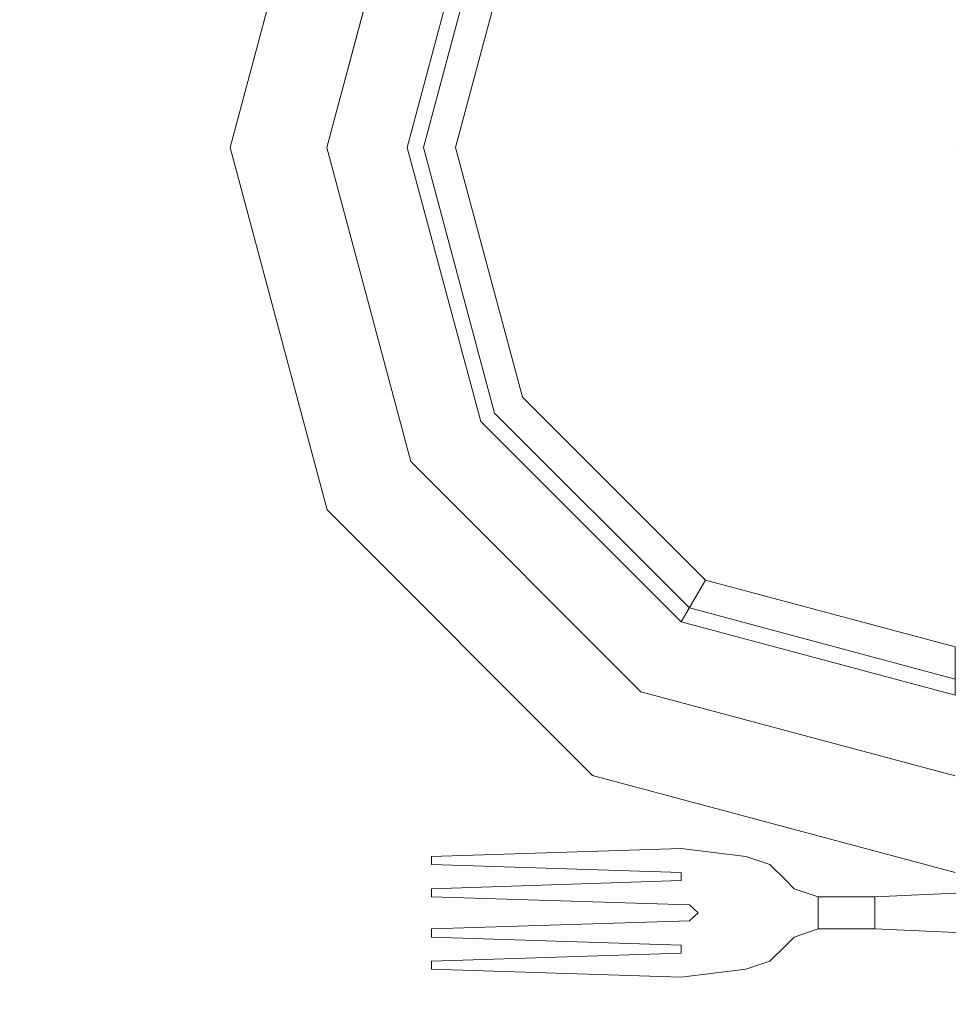
# Model space of a CAD drawing. Units: inches. Extents: x 375 to 1122, y 27 to 1069.
# Tile 55 of 155: x 732.625 to 739.718, y 296.542 to 304.063. Entities that reach past the tile are written whole.
import ezdxf

# ---------------------------------------------------------------- set-up
doc = ezdxf.new("R2010")
doc.units = ezdxf.units.IN
doc.layers.add('A-ANNO-DIMS', color=2, linetype='Continuous', lineweight=18)
doc.layers.add('Furniture', color=30, linetype='Continuous', lineweight=18)
doc.styles.get("Standard").update_dxf_attribs({"font": 'arial.ttf'})
doc.dimstyles.new('ISO-25', dxfattribs={"dimtxt": 12, "dimasz": 2.5, "dimexe": 1.5, "dimexo": 1.5, "dimtad": 1, "dimdec": 1, "dimlunit": 3, "dimtxsty": 'Standard', "dimblk": 'ARCHTICK', "dimcen": 2.5, "dimadec": 0, "dimazin": 0, "dimtfac": 1, "dimtdec": 1, "dimtmove": 0, "dimatfit": 3, "dimfxl": 1.5, "dimfxlon": 1, "dimarcsym": 0})

# ---------------------------------------------------------------- blocks, each defined once
blk = doc.blocks.new('A$C403C54AD')
for p, q in [((1.2372, 1.33067, -0.03581), (1.23566, 1.33529, -0.03534)), ((1.2372, 1.33067, -0.03888), (1.23566, 1.33529, -0.03842))]:
    blk.add_line(p, q)
for points, invisible_edges in [([(1.22181, 1.3907, -0.03153), (1.23105, 1.3907, -0.03153), (1.22951, 1.3553, -0.02863), (1.22335, 1.3553, -0.02863)], 1), ([(1.22181, 1.3907, -0.03153), (1.22181, 1.3907, -0.03461), (1.22335, 1.3553, -0.03122), (1.22335, 1.3553, -0.02863)], 5), ([(1.22181, 1.3907, -0.03461), (1.23105, 1.3907, -0.03461), (1.22951, 1.3553, -0.03122), (1.22335, 1.3553, -0.03122)], 1), ([(1.22951, 1.3553, -0.02863), (1.22951, 1.3553, -0.03122), (1.23105, 1.3907, -0.03461), (1.23105, 1.3907, -0.03153)], 5), ([(1.22335, 1.3553, -0.03122), (1.22335, 1.3553, -0.02863), (1.22335, 1.34452, -0.03071), (1.22335, 1.34452, -0.0333)], 5), ([(1.22951, 1.34452, -0.0333), (1.22951, 1.34452, -0.03071), (1.22951, 1.3553, -0.02863), (1.22951, 1.3553, -0.03122)], 5), ([(1.22335, 1.34452, -0.03071), (1.22951, 1.34452, -0.03071), (1.23105, 1.33991, -0.03306), (1.22181, 1.33991, -0.03306)], 4), ([(1.22335, 1.34452, -0.03071), (1.22335, 1.34452, -0.0333), (1.22181, 1.33991, -0.03584), (1.22181, 1.33991, -0.03306)], 5), ([(1.22335, 1.34452, -0.0333), (1.22951, 1.34452, -0.0333), (1.23105, 1.33991, -0.03584), (1.22181, 1.33991, -0.03584)], 4), ([(1.22951, 1.34452, -0.0333), (1.22951, 1.34452, -0.03071), (1.23105, 1.33991, -0.03306), (1.23105, 1.33991, -0.03584)], 5), ([(1.23105, 1.33991, -0.03306), (1.22181, 1.33991, -0.03306), (1.22027, 1.33837, -0.0341), (1.23258, 1.33837, -0.0341)], 5), ([(1.23105, 1.33991, -0.03584), (1.22181, 1.33991, -0.03584), (1.22027, 1.33837, -0.03718), (1.23258, 1.33837, -0.03718)], 5), ([(1.22181, 1.33991, -0.03584), (1.22181, 1.33991, -0.03306), (1.22027, 1.33837, -0.0341), (1.22027, 1.33837, -0.03718)], 1), ([(1.23105, 1.33991, -0.03306), (1.23105, 1.33991, -0.03584), (1.23258, 1.33837, -0.03718), (1.23258, 1.33837, -0.0341)], 1), ([(1.23258, 1.33837, -0.03718), (1.22027, 1.33837, -0.03718), (1.21719, 1.33529, -0.03842), (1.23566, 1.33529, -0.03842)], 5), ([(1.23258, 1.33837, -0.0341), (1.22027, 1.33837, -0.0341), (1.21719, 1.33529, -0.03534), (1.23566, 1.33529, -0.03534)], 5), ([(1.21719, 1.33529, -0.03534), (1.23566, 1.33529, -0.03534), (1.2372, 1.33067, -0.03581), (1.21565, 1.33067, -0.03581)], 5), ([(1.21719, 1.33529, -0.03842), (1.23566, 1.33529, -0.03842), (1.2372, 1.33067, -0.03888), (1.21565, 1.33067, -0.03888)], 5), ([(1.21719, 1.33529, -0.03842), (1.21719, 1.33529, -0.03534), (1.21565, 1.33067, -0.03581), (1.21565, 1.33067, -0.03888)], 4), ([(1.23566, 1.33529, -0.03534), (1.23566, 1.33529, -0.03842), (1.2372, 1.33067, -0.03888), (1.2372, 1.33067, -0.03581)], 4), ([(1.21565, 1.33067, -0.03581), (1.22027, 1.31836, -0.03521), (1.21873, 1.31836, -0.03521), (1.21411, 1.31836, -0.03521)], 5), ([(1.21565, 1.33067, -0.03888), (1.22027, 1.31836, -0.03829), (1.21873, 1.31836, -0.03829), (1.21411, 1.31836, -0.03829)], 5), ([(1.21565, 1.33067, -0.03581), (1.21565, 1.33067, -0.03888), (1.21411, 1.31836, -0.03829), (1.21411, 1.31836, -0.03521)], 1), ([(1.21565, 1.33067, -0.03581), (1.22643, 1.32156, -0.0356), (1.22489, 1.3199, -0.03545), (1.22027, 1.31836, -0.03521)], 13), ([(1.21565, 1.33067, -0.03581), (1.22643, 1.32156, -0.0356), (1.2372, 1.33067, -0.03581), (1.21565, 1.33067, -0.03581)], 7), ([(1.21565, 1.33067, -0.03888), (1.22643, 1.32156, -0.03868), (1.2372, 1.33067, -0.03888), (1.21565, 1.33067, -0.03888)], 7), ([(1.21565, 1.33067, -0.03888), (1.22643, 1.32156, -0.03868), (1.22489, 1.3199, -0.03853), (1.22027, 1.31836, -0.03829)], 13), ([(1.2372, 1.33067, -0.03581), (1.22643, 1.32156, -0.0356), (1.22797, 1.3199, -0.03545), (1.23258, 1.31836, -0.03521)], 13), ([(1.2372, 1.33067, -0.03888), (1.22643, 1.32156, -0.03868), (1.22797, 1.3199, -0.03853), (1.23258, 1.31836, -0.03829)], 13), ([(1.2372, 1.33067, -0.03581), (1.23258, 1.31836, -0.03521), (1.23412, 1.31836, -0.03521), (1.23874, 1.31836, -0.03521)], 5), ([(1.2372, 1.33067, -0.03888), (1.23258, 1.31836, -0.03829), (1.23412, 1.31836, -0.03829), (1.23874, 1.31836, -0.03829)], 5), ([(1.2372, 1.33067, -0.03888), (1.2372, 1.33067, -0.03581), (1.23874, 1.31836, -0.03521), (1.23874, 1.31836, -0.03829)], 1), ([(1.22027, 1.31836, -0.03521), (1.22489, 1.3199, -0.03545), (1.22335, 1.27064, -0.02811), (1.22181, 1.27064, -0.02811)], 1), ([(1.22027, 1.31836, -0.03829), (1.22489, 1.3199, -0.03853), (1.22335, 1.27064, -0.03119), (1.22181, 1.27064, -0.03119)], 1), ([(1.22797, 1.3199, -0.03545), (1.23258, 1.31836, -0.03521), (1.23105, 1.27064, -0.02811), (1.22951, 1.27064, -0.02811)], 1), ([(1.22797, 1.3199, -0.03853), (1.23258, 1.31836, -0.03829), (1.23105, 1.27064, -0.03119), (1.22951, 1.27064, -0.03119)], 1), ([(1.21873, 1.31836, -0.03521), (1.21411, 1.31836, -0.03521), (1.21565, 1.27064, -0.02811), (1.21719, 1.27064, -0.02811)], 1), ([(1.21873, 1.31836, -0.03829), (1.21411, 1.31836, -0.03829), (1.21565, 1.27064, -0.03119), (1.21719, 1.27064, -0.03119)], 1), ([(1.23412, 1.31836, -0.03521), (1.23874, 1.31836, -0.03521), (1.2372, 1.27064, -0.02811), (1.23566, 1.27064, -0.02811)], 1), ([(1.23412, 1.31836, -0.03829), (1.23874, 1.31836, -0.03829), (1.2372, 1.27064, -0.03119), (1.23566, 1.27064, -0.03119)], 1)]:
    blk.add_3dface(points, dxfattribs=dict(invisible_edges=invisible_edges))
at = {"linetype": 'ByBlock'}
for points, invisible_edges in [([(0.97862, 1.37069, -0.02965), (1.0802, 1.37069, -0.02965), (1.0802, 1.37069, -0.02965), (0.99223, 1.3199, -0.02965)], 5), ([(0.99223, 1.3199, -0.02965), (1.0802, 1.37069, -0.02965), (1.0802, 1.37069, -0.02965), (1.02941, 1.28271, -0.02965)], 5), ([(1.02941, 1.28271, -0.02965), (1.0802, 1.37069, -0.02965), (1.0802, 1.37069, -0.02965), (1.0802, 1.2691, -0.02965)], 5), ([(1.0802, 1.2691, -0.02965), (1.0802, 1.37069, -0.02965), (1.0802, 1.37069, -0.02965), (1.131, 1.28271, -0.02965)], 5), ([(1.16818, 1.3199, -0.02965), (1.0802, 1.37069, -0.02965), (1.0802, 1.37069, -0.02965), (1.18179, 1.37069, -0.02965)], 5), ([(1.131, 1.28271, -0.02965), (1.0802, 1.37069, -0.02965), (1.0802, 1.37069, -0.02965), (1.16818, 1.3199, -0.02965)], 5), ([(1.18418, 1.31066, -0.02349), (1.16818, 1.3199, -0.02965), (1.18179, 1.37069, -0.02965), (1.20026, 1.37069, -0.02349)], 5), ([(1.17085, 1.31836, -0.03734), (1.20017, 1.30143, -0.02811), (1.21873, 1.37069, -0.02811), (1.18487, 1.37069, -0.03734)], 5), ([(1.20017, 1.30143, -0.02349), (1.18418, 1.31066, -0.02349), (1.20026, 1.37069, -0.02349), (1.21873, 1.37069, -0.02349)], 5), ([(1.12792, 1.28804, -0.04658), (1.13254, 1.28005, -0.03734), (1.17085, 1.31836, -0.03734), (1.16285, 1.32297, -0.04658)], 1), ([(1.14023, 1.26672, -0.02349), (1.131, 1.28271, -0.02965), (1.16818, 1.3199, -0.02965), (1.18418, 1.31066, -0.02349)], 5), ([(1.13254, 1.28005, -0.03734), (1.14947, 1.25072, -0.02811), (1.20017, 1.30143, -0.02811), (1.17085, 1.31836, -0.03734)], 5), ([(1.14947, 1.25072, -0.02349), (1.14023, 1.26672, -0.02349), (1.18418, 1.31066, -0.02349), (1.20017, 1.30143, -0.02349)], 5), ([(1.03249, 1.28804, -0.04658), (1.02787, 1.28005, -0.03734), (1.0802, 1.26602, -0.03734), (1.0802, 1.27526, -0.04658)], 5), ([(1.0802, 1.27526, -0.04658), (1.0802, 1.26602, -0.03734), (1.13254, 1.28005, -0.03734), (1.12792, 1.28804, -0.04658)], 5), ([(1.02018, 1.26672, -0.02349), (1.02941, 1.28271, -0.02965), (1.0802, 1.2691, -0.02965), (1.0802, 1.25063, -0.02349)], 5), ([(1.0802, 1.25063, -0.02349), (1.0802, 1.2691, -0.02965), (1.131, 1.28271, -0.02965), (1.14023, 1.26672, -0.02349)], 5), ([(1.02787, 1.28005, -0.03734), (1.01094, 1.25072, -0.02811), (1.0802, 1.23216, -0.02811), (1.0802, 1.26602, -0.03734)], 5), ([(1.0802, 1.26602, -0.03734), (1.0802, 1.23216, -0.02811), (1.14947, 1.25072, -0.02811), (1.13254, 1.28005, -0.03734)], 5), ([(1.01094, 1.25072, -0.02349), (1.02018, 1.26672, -0.02349), (1.0802, 1.25063, -0.02349), (1.0802, 1.23216, -0.02349)], 5), ([(1.0802, 1.23216, -0.02349), (1.0802, 1.25063, -0.02349), (1.14023, 1.26672, -0.02349), (1.14947, 1.25072, -0.02349)], 5)]:
    blk.add_3dface(points, dxfattribs=dict(at, invisible_edges=invisible_edges))
for points in [[(1.16285, 1.32297, -0.04658), (1.17085, 1.31836, -0.03734), (1.18487, 1.37069, -0.03734), (1.17563, 1.37069, -0.04658)], [(1.20017, 1.30143, -0.02811), (1.20017, 1.30143, -0.02349), (1.21873, 1.37069, -0.02349), (1.21873, 1.37069, -0.02811)], [(1.14947, 1.25072, -0.02811), (1.14947, 1.25072, -0.02349), (1.20017, 1.30143, -0.02349), (1.20017, 1.30143, -0.02811)], [(1.01094, 1.25072, -0.02811), (1.01094, 1.25072, -0.02349), (1.0802, 1.23216, -0.02349), (1.0802, 1.23216, -0.02811)], [(1.0802, 1.23216, -0.02811), (1.0802, 1.23216, -0.02349), (1.14947, 1.25072, -0.02349), (1.14947, 1.25072, -0.02811)]]:
    blk.add_3dface(points, dxfattribs=at)
for points in [[(1.22951, 1.3553, -0.02863), (1.22335, 1.3553, -0.02863), (1.22335, 1.34452, -0.03071), (1.22951, 1.34452, -0.03071)], [(1.22951, 1.3553, -0.03122), (1.22335, 1.3553, -0.03122), (1.22335, 1.34452, -0.0333), (1.22951, 1.34452, -0.0333)], [(1.22027, 1.33837, -0.0341), (1.22027, 1.33837, -0.03718), (1.21719, 1.33529, -0.03842), (1.21719, 1.33529, -0.03534)], [(1.23258, 1.33837, -0.03718), (1.23258, 1.33837, -0.0341), (1.23566, 1.33529, -0.03534), (1.23566, 1.33529, -0.03842)], [(1.22643, 1.32156, -0.03868), (1.22643, 1.32156, -0.0356), (1.22489, 1.3199, -0.03545), (1.22489, 1.3199, -0.03853)], [(1.22797, 1.3199, -0.03545), (1.22797, 1.3199, -0.03853), (1.22643, 1.32156, -0.03868), (1.22643, 1.32156, -0.0356)], [(1.22335, 1.27064, -0.03119), (1.22335, 1.27064, -0.02811), (1.22489, 1.3199, -0.03545), (1.22489, 1.3199, -0.03853)], [(1.22797, 1.3199, -0.03853), (1.22797, 1.3199, -0.03545), (1.22951, 1.27064, -0.02811), (1.22951, 1.27064, -0.03119)], [(1.21411, 1.31836, -0.03829), (1.21411, 1.31836, -0.03521), (1.21565, 1.27064, -0.02811), (1.21565, 1.27064, -0.03119)], [(1.21719, 1.27064, -0.02811), (1.21719, 1.27064, -0.03119), (1.21873, 1.31836, -0.03829), (1.21873, 1.31836, -0.03521)], [(1.22027, 1.31836, -0.03829), (1.22027, 1.31836, -0.03521), (1.21873, 1.31836, -0.03521), (1.21873, 1.31836, -0.03829)], [(1.22027, 1.31836, -0.03829), (1.22027, 1.31836, -0.03521), (1.22181, 1.27064, -0.02811), (1.22181, 1.27064, -0.03119)], [(1.23105, 1.27064, -0.02811), (1.23105, 1.27064, -0.03119), (1.23258, 1.31836, -0.03829), (1.23258, 1.31836, -0.03521)], [(1.23412, 1.31836, -0.03521), (1.23412, 1.31836, -0.03829), (1.23258, 1.31836, -0.03829), (1.23258, 1.31836, -0.03521)], [(1.23412, 1.31836, -0.03521), (1.23412, 1.31836, -0.03829), (1.23566, 1.27064, -0.03119), (1.23566, 1.27064, -0.02811)], [(1.2372, 1.27064, -0.02811), (1.2372, 1.27064, -0.03119), (1.23874, 1.31836, -0.03829), (1.23874, 1.31836, -0.03521)], [(1.21565, 1.27064, -0.03119), (1.21565, 1.27064, -0.02811), (1.21719, 1.27064, -0.02811), (1.21719, 1.27064, -0.03119)], [(1.22181, 1.27064, -0.03119), (1.22181, 1.27064, -0.02811), (1.22335, 1.27064, -0.02811), (1.22335, 1.27064, -0.03119)], [(1.22951, 1.27064, -0.03119), (1.22951, 1.27064, -0.02811), (1.23105, 1.27064, -0.02811), (1.23105, 1.27064, -0.03119)], [(1.23566, 1.27064, -0.03119), (1.23566, 1.27064, -0.02811), (1.2372, 1.27064, -0.02811), (1.2372, 1.27064, -0.03119)]]:
    blk.add_3dface(points)
blk = doc.blocks.new('_ArchTick')
at = {"color": 0, "linetype": 'ByBlock', "const_width": 0.15}
blk.add_lwpolyline([(-0.5, -0.5), (0.5, 0.5)], dxfattribs=at)
blk = doc.blocks.new('*D94')
at = {"layer": 'A-ANNO-DIMS', "color": 0, "lineweight": -2, "transparency": 16777216}
for p, q in [((734.0073, 117.5277), (734.0073, 114.5277)), ((773.0073, 117.5277), (773.0073, 114.5277)), ((734.0073, 116.0277), (773.0073, 116.0277))]:
    blk.add_line(p, q, dxfattribs=at)
at = {"layer": 'Defpoints', "color": 0, "transparency": 16777216}
for p in [(734.0073, 667.5277), (773.0073, 667.5277), (773.0073, 116.0277)]:
    blk.add_point(p, dxfattribs=at)
at = {"layer": 'A-ANNO-DIMS', "color": 0, "lineweight": -2, "transparency": 16777216, "xscale": 2.5, "yscale": 2.5, "zscale": 2.5, "rotation": 180}
blk.add_blockref('_ArchTick', (734.0073, 116.0277), dxfattribs=at)
at = {"layer": 'A-ANNO-DIMS', "color": 0, "lineweight": -2, "transparency": 16777216, "xscale": 2.5, "yscale": 2.5, "zscale": 2.5}
blk.add_blockref('_ArchTick', (773.0073, 116.0277), dxfattribs=at)
at = {"layer": 'A-ANNO-DIMS', "color": 0, "transparency": 16777216, "insert": (753.5073, 122.7837), "char_height": 12, "attachment_point": 5}
blk.add_mtext('3\'-3"', dxfattribs=at)

msp = doc.modelspace()

# ---------------------------------------------------------------- block references
at = {"layer": 'Furniture', "xscale": 39.9918517141215, "yscale": 39.9918517141215, "zscale": 39.9918517141215, "rotation": 270}
msp.add_blockref('A$C403C54AD', (684.9549, 346.2875, 0.024), dxfattribs=at)

# ---------------------------------------------------------------- dimensions: what is measured, and where the dimension line sits
at = {"layer": 'A-ANNO-DIMS'}
dim = msp.add_linear_dim(base=(773.0073, 116.0277), p1=(734.0073, 667.5277), p2=(773.0073, 667.5277), dimstyle='ISO-25', override={"dimdec": 1, "dimlfac": 1, "dimrnd": 0, "dimzin": 1, "dimdsep": 46, "dimlunit": 4, "dimfrac": 2}, dxfattribs=at)
dim.commit()
dim.dimension.update_dxf_attribs({"geometry": '*D94', "text_midpoint": (753.5073, 122.7837)})

doc.saveas('drawing.dxf')
